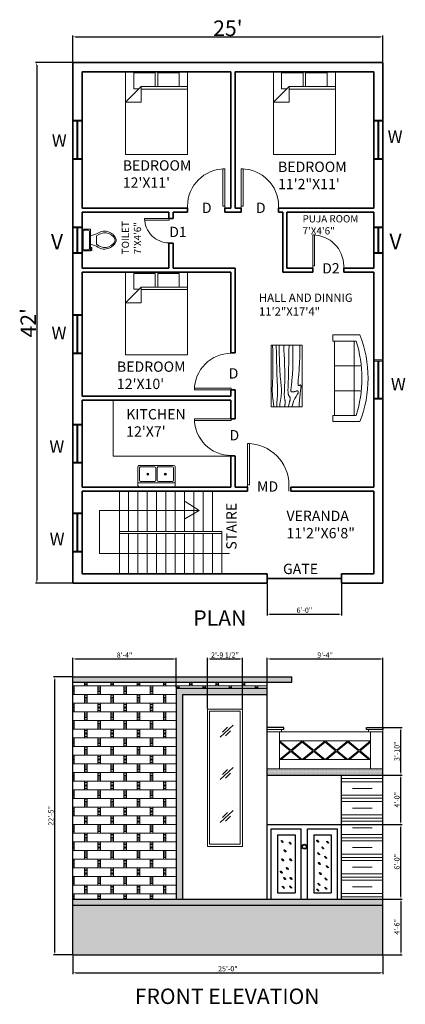
# Model space of a CAD drawing. Units: inches. Extents: x 1662 to 23131, y 1265 to 19127.
# Tile 5 of 26: x 10200 to 10573, y 5334 to 6287. Entities that reach past the tile are written whole.
import ezdxf

# ---------------------------------------------------------------- set-up
doc = ezdxf.new("R2010")
doc.units = ezdxf.units.IN
for name, color, linetype, lineweight in [('A-ANNO-DIMS', 4, 'Continuous', 18), ('A-ANNO-IDEN', 7, 'Continuous', 18), ('A-ANNO-TITL', 7, 'Continuous', 35), ('A-AREA-IDEN', 7, 'Continuous', 18), ('A-DOOR', 3, 'Continuous', 18), ('A-ELEV', 7, 'Continuous', 25), ('A-ELEV-GLAZ', 4, 'Continuous', 18), ('A-ELEV-PATT', 8, 'Continuous', 13), ('A-ELEV-RAIL', 7, 'Continuous', 18), ('A-ELEV-SURF-PATT', 252, 'Continuous', 13), ('A-FLOR-CASE', 8, 'Continuous', 18), ('A-FLOR-FIXT', 9, 'Continuous', 18), ('A-FLOR-STRS', 7, 'Continuous', 18), ('A-FURN', 8, 'Continuous', 18), ('A-GLAZ', 4, 'Continuous', 18), ('A-WALL', 7, 'Continuous', 35)]:
    doc.layers.add(name, color=color, linetype=linetype, lineweight=lineweight)
doc.styles.get("Standard").update_dxf_attribs({"font": 'arial.ttf'})
doc.dimstyles.new('ISO-25', dxfattribs={"dimtxt": 5, "dimasz": 2.5, "dimexe": 1.25, "dimexo": 0.625, "dimtad": 1, "dimlunit": 3, "dimtxsty": 'Standard', "dimcen": 2.5, "dimadec": 0, "dimazin": 0, "dimtfac": 1, "dimtmove": 0, "dimatfit": 3, "dimfxl": 1, "dimarcsym": 0})
pattern_1 = [(0, (-2241.2752, 386.7928), (0.79375, 1.5875), [0, -1.5875])]

# ---------------------------------------------------------------- blocks, each defined once
blk = doc.blocks.new('Bed - Queen')
for p, q in [((0, -80.00003), (0, 0)), ((0, 0), (59.99999, 0)), ((59.99999, 0), (59.99999, -80.00003)), ((7.99999, -1.2), (28.79998, -1.2)), ((7.99999, -14.4), (7.99999, -1.2)), ((28.79998, -1.2), (28.79998, -14.4)), ((31.19999, -1.2), (51.99999, -1.2)), ((31.19999, -14.4), (31.19999, -1.2)), ((51.99999, -1.2), (51.99999, -16.4)), ((0, -14.4), (44.8, -14.4)), ((44.8, -16.8), (0, -16.8)), ((59.99999, -29.6), (44.8, -14.4)), ((44.8, -14.4), (44.8, -29.6)), ((51.99999, -16.4), (46.79936, -16.4)), ((44.8, -29.6), (59.99999, -29.6)), ((59.99999, -80.00003), (0, -80.00003))]:
    blk.add_line(p, q)
blk = doc.blocks.new('Table - Rectangular Woodgrain 60 x 30 in.')
for p, q in [((0, 0), (0, -30)), ((60, 0), (0, 0)), ((60, -30), (60, 0)), ((0, -30), (60, -30))]:
    blk.add_line(p, q)
for points in [[(0, -2.4), (4.8155, -2.418), (9.0302, -2.4688), (12.709, -2.5477), (15.9167, -2.65), (18.7181, -2.7711), (21.1781, -2.9063), (23.3616, -3.0508), (25.3333, -3.2), (27.1477, -3.3495), (28.8172, -3.4958), (30.3437, -3.636), (31.7291, -3.7667), (32.9756, -3.8849), (34.0849, -3.9875), (35.059, -4.0714), (35.9, -4.1334), (36.6114, -4.1711), (37.2041, -4.1854), (37.6906, -4.1779), (38.0833, -4.15), (38.3948, -4.1034), (38.6375, -4.0396), (38.8239, -3.9602), (38.9666, -3.8667), (39.0764, -3.7608), (39.1573, -3.6448), (39.2116, -3.521), (39.2416, -3.3917), (39.2498, -3.2593), (39.2385, -3.1261), (39.21, -2.9944), (39.1666, -2.8667), (39.111, -2.7447), (39.0468, -2.6281), (38.978, -2.5163), (38.9083, -2.4083), (38.8418, -2.3035), (38.7823, -2.201), (38.7337, -2.1001), (38.7, -2), (38.6844, -1.9003), (38.6875, -1.8021), (38.7094, -1.707), (38.75, -1.6167), (38.8094, -1.5326), (38.8875, -1.4563), (38.9844, -1.3893), (39.1, -1.3333), (39.2351, -1.2896), (39.3937, -1.2583), (39.5804, -1.2396), (39.8, -1.2333), (40.057, -1.2396), (40.3562, -1.2583), (40.7023, -1.2896), (41.1, -1.3333), (41.5547, -1.3895), (42.0755, -1.4573), (42.6721, -1.5361), (43.3542, -1.625), (44.1316, -1.7233), (45.014, -1.8302), (46.0114, -1.9449), (47.1333, -2.0667), (48.3862, -2.1947), (49.7625, -2.3281), (51.2513, -2.4663), (52.8416, -2.6083), (54.5226, -2.7535), (56.2833, -2.9011), (58.1127, -3.0501), (60, -3.2)], [(0, -9.2), (6.5759, -9.0858), (11.9385, -9.0365), (16.2527, -9.0418), (19.6833, -9.0917), (22.3952, -9.1759), (24.5531, -9.2844), (26.322, -9.4069), (27.8666, -9.5333), (29.3241, -9.6553), (30.7203, -9.7719), (32.0532, -9.8837), (33.3208, -9.9917), (34.5213, -10.0965), (35.6526, -10.199), (36.7128, -10.2999), (37.7, -10.4), (38.6129, -10.4996), (39.4531, -10.5969), (40.223, -10.6895), (40.925, -10.775), (41.5613, -10.8512), (42.1344, -10.9156), (42.6465, -10.966), (43.1, -11), (43.4976, -11.0158), (43.8437, -11.0136), (44.143, -10.9942), (44.4, -10.9583), (44.6195, -10.9069), (44.8062, -10.8406), (44.9648, -10.7603), (45.1, -10.6667), (45.2155, -10.5598), (45.3114, -10.4365), (45.3871, -10.2929), (45.4416, -10.125), (45.4743, -9.929), (45.4844, -9.7011), (45.4709, -9.4371), (45.4333, -9.1333), (45.3716, -8.7883), (45.2896, -8.4104), (45.1919, -8.0107), (45.0833, -7.6), (44.9685, -7.1893), (44.8521, -6.7896), (44.7388, -6.4117), (44.6333, -6.0667), (44.54, -5.7628), (44.4614, -5.4979), (44.4001, -5.2675), (44.3583, -5.0667), (44.3384, -4.8909), (44.3427, -4.7354), (44.3736, -4.5956), (44.4333, -4.4667), (44.5236, -4.3453), (44.6427, -4.2333), (44.7884, -4.1339), (44.9583, -4.05), (45.1501, -3.9849), (45.3614, -3.9417), (45.59, -3.9234), (45.8333, -3.9333), (46.0915, -3.9749), (46.3734, -4.0531), (46.6906, -4.1736), (47.0542, -4.3417), (47.4756, -4.5629), (47.9661, -4.8427), (48.5372, -5.1866), (49.2, -5.6), (49.9676, -6.0844), (50.8594, -6.625), (51.8965, -7.2031), (53.1, -7.8), (54.491, -8.3969), (56.0906, -8.975), (57.9199, -9.5156), (60, -10)], [(0, -12.8), (5.1847, -12.9322), (9.6213, -13.0323), (13.3963, -13.1059), (16.5958, -13.1583), (19.3063, -13.1952), (21.614, -13.2219), (23.6054, -13.2439), (25.3666, -13.2667), (26.9728, -13.2947), (28.4531, -13.3281), (29.8256, -13.3663), (31.1083, -13.4083), (32.3191, -13.4535), (33.476, -13.501), (34.597, -13.5501), (35.7, -13.6), (36.7984, -13.6497), (37.8875, -13.6979), (38.9578, -13.743), (40, -13.7833), (41.0047, -13.8174), (41.9625, -13.8438), (42.864, -13.8607), (43.7, -13.8667), (44.4631, -13.8604), (45.1552, -13.8417), (45.7801, -13.8104), (46.3416, -13.7667), (46.8439, -13.7104), (47.2906, -13.6417), (47.6858, -13.5604), (48.0333, -13.4667), (48.3375, -13.3608), (48.6042, -13.2448), (48.8396, -13.121), (49.05, -12.9917), (49.2417, -12.8593), (49.4208, -12.7261), (49.5937, -12.5944), (49.7667, -12.4667), (49.9452, -12.3451), (50.1323, -12.2313), (50.3303, -12.1268), (50.5416, -12.0333), (50.7686, -11.9524), (51.0135, -11.8854), (51.2788, -11.8341), (51.5666, -11.8), (51.8785, -11.7843), (52.2116, -11.7865), (52.562, -11.8059), (52.926, -11.8417), (53.2998, -11.8931), (53.6795, -11.9594), (54.0614, -12.0397), (54.4416, -12.1333), (54.8223, -12.2401), (55.2293, -12.3625), (55.6942, -12.5037), (56.2489, -12.6667), (56.9251, -12.8547), (57.7545, -13.0708), (58.7689, -13.3182), (60, -13.6)], [(0, -18), (5.124, -17.7273), (9.6609, -17.5057), (13.6705, -17.3303), (17.2125, -17.1958), (20.3467, -17.0973), (23.1328, -17.0297), (25.6307, -16.9878), (27.9, -16.9667), (29.9928, -16.9617), (31.9302, -16.9703), (33.7254, -16.9907), (35.3917, -17.0208), (36.9423, -17.0588), (38.3906, -17.1026), (39.7499, -17.1503), (41.0333, -17.2), (42.2519, -17.2496), (43.4073, -17.2969), (44.4986, -17.3395), (45.525, -17.375), (46.4858, -17.4012), (47.3802, -17.4156), (48.2074, -17.416), (48.9667, -17.4), (49.6583, -17.3662), (50.2872, -17.3167), (50.8595, -17.2547), (51.3812, -17.1833), (51.8584, -17.1057), (52.2971, -17.025), (52.7034, -16.9443), (53.0833, -16.8667), (53.443, -16.7951), (53.789, -16.7313), (54.128, -16.6768), (54.4666, -16.6334), (54.8115, -16.6024), (55.1693, -16.5854), (55.5465, -16.5841), (55.95, -16.6), (56.3828, -16.6337), (56.8346, -16.6823), (57.2915, -16.7418), (57.7396, -16.8084), (58.165, -16.878), (58.5539, -16.9469), (58.8924, -17.0111), (59.1666, -17.0667), (59.3679, -17.1107), (59.5078, -17.1438), (59.6032, -17.1675), (59.6708, -17.1833), (59.7275, -17.193), (59.7901, -17.1979), (59.8753, -17.1998), (60, -17.2)], [(0, -22.4), (8.0098, -22.2501), (14.4094, -22.1011), (19.4168, -21.9535), (23.25, -21.8083), (26.1269, -21.6663), (28.2656, -21.5281), (29.884, -21.3947), (31.2, -21.2667), (32.3967, -21.1448), (33.5172, -21.0292), (34.5697, -20.9198), (35.5625, -20.8167), (36.5037, -20.7198), (37.4015, -20.6292), (38.2642, -20.5448), (39.1, -20.4667), (39.9164, -20.3951), (40.7187, -20.3313), (41.5117, -20.2768), (42.3, -20.2333), (43.0883, -20.2024), (43.8812, -20.1854), (44.6836, -20.1841), (45.5, -20.2), (46.3328, -20.234), (47.1747, -20.2844), (48.0163, -20.3488), (48.8479, -20.425), (49.66, -20.5106), (50.4429, -20.6031), (51.1872, -20.7004), (51.8833, -20.8), (52.5246, -20.8999), (53.1166, -20.9995), (53.6681, -21.0983), (54.1875, -21.1958), (54.6834, -21.2919), (55.1646, -21.3859), (55.6394, -21.4777), (56.1167, -21.5667), (56.6028, -21.6515), (57.0961, -21.7266), (57.5929, -21.7852), (58.0896, -21.8208), (58.5823, -21.8268), (59.0674, -21.7964), (59.5412, -21.723), (60, -21.6)], [(0, -25.2), (8.6355, -25.0504), (15.7026, -24.9031), (21.4049, -24.7606), (25.9458, -24.625), (29.529, -24.4988), (32.3578, -24.3844), (34.6359, -24.284), (36.5667, -24.2), (38.3213, -24.1341), (39.9417, -24.0854), (41.437, -24.0523), (42.8167, -24.0333), (44.0901, -24.0268), (45.2667, -24.0313), (46.3557, -24.0451), (47.3667, -24.0667), (48.309, -24.0947), (49.1928, -24.1287), (50.0284, -24.168), (50.826, -24.2125), (51.5959, -24.2617), (52.3483, -24.3151), (53.0935, -24.3725), (53.8417, -24.4334), (54.6009, -24.497), (55.3699, -24.561), (56.1454, -24.6226), (56.9239, -24.6792), (57.7021, -24.7279), (58.4764, -24.7662), (59.2435, -24.7911), (60, -24.8)], [(0, -28.8), (5.6867, -28.6681), (10.45, -28.5698), (14.407, -28.5012), (17.675, -28.4584), (20.3711, -28.4374), (22.6125, -28.4344), (24.5164, -28.4455), (26.2, -28.4667), (27.762, -28.4947), (29.2276, -28.5281), (30.6033, -28.5663), (31.8958, -28.6084), (33.1118, -28.6535), (34.2578, -28.7011), (35.3405, -28.7501), (36.3666, -28.8), (37.3443, -28.8497), (38.288, -28.8974), (39.2137, -28.9412), (40.1375, -28.9792), (41.0753, -29.0093), (42.0432, -29.0297), (43.0572, -29.0384), (44.1333, -29.0333), (45.2936, -29.0114), (46.5843, -28.9641), (48.0579, -28.8816), (49.7666, -28.7542), (51.7629, -28.5721), (54.0989, -28.3255), (56.8272, -28.0048), (60, -27.6)]]:
    blk.add_lwpolyline(points)
blk = doc.blocks.new('Sofa - Roundback 7 ft.')
for p, q in [((-12.00002, -32.4421), (-12.00003, -6.5971)), ((11.99997, -32.4421), (11.99998, -6.5971)), ((-36.000027, -34), (-36.000027, -11.4696)), ((-35.999844, -13.3819), (35.9998, -13.3819)), ((35.99998, -34), (35.99998, -11.4696)), ((-36.000027, -32.4421), (35.99998, -32.4421))]:
    blk.add_line(p, q)
for points in [[(-36.000027, -34), (-42.000027, -34), (-42.000027, -8)], [(41.99998, -8), (41.99998, -34), (35.99998, -34)]]:
    blk.add_lwpolyline(points)
for centre, radius, start, end in [((0, -114.25), 114.25, 68.43141, 111.5686), ((-0.00001, -127.1968), 121.1968, 72.72033, 107.2797)]:
    blk.add_arc(centre, radius, start, end)
blk = doc.blocks.new('*U34')
for p, q in [((0, 0), (0, -6)), ((-36, 0), (-36, -6))]:
    blk.add_line(p, q)
blk.add_lwpolyline([(0, 0), (0, 36), (-1.75, 36), (-1.75, 0)], close=True)
blk.add_arc((0, 0), 36, 90, 180)
blk = doc.blocks.new('*U46')
for p, q in [((0, 0), (0, -6)), ((36, 0), (36, -6))]:
    blk.add_line(p, q)
blk.add_lwpolyline([(0, 0), (0, 36), (1.75, 36), (1.75, 0)], close=True)
blk.add_arc((0, 0), 36, 0, 90)
blk = doc.blocks.new('*U41')
for p, q in [((0, 0), (0, -100)), ((-900, 0), (-900, -100))]:
    blk.add_line(p, q)
blk.add_lwpolyline([(0, 0), (0, 900), (-43.75, 900), (-43.75, 0)], close=True)
blk.add_arc((0, 0), 900, 90, 180)
blk = doc.blocks.new('*U42')
for p, q in [((0, 0), (0, -100)), ((900, 0), (900, -100))]:
    blk.add_line(p, q)
blk.add_lwpolyline([(0, 0), (0, 900), (43.75, 900), (43.75, 0)], close=True)
blk.add_arc((0, 0), 900, 0, 90)
blk = doc.blocks.new('*U33')
for p, q in [((0, 0), (0, -6)), ((40, 0), (40, -6))]:
    blk.add_line(p, q)
blk.add_lwpolyline([(0, 0), (0, 40), (1.75, 40), (1.75, 0)], close=True)
blk.add_arc((0, 0), 40, 0, 90)
blk = doc.blocks.new('*U47')
for p, q in [((0, 0), (0, -6)), ((30, 0), (30, -6))]:
    blk.add_line(p, q)
blk.add_lwpolyline([(0, 0), (0, 30), (1.75, 30), (1.75, 0)], close=True)
blk.add_arc((0, 0), 30, 0, 90)
blk = doc.blocks.new('*U48')
for p, q in [((0, 0), (0, 100)), ((600, 0), (600, 100))]:
    blk.add_line(p, q)
blk.add_lwpolyline([(0, 0), (0, -600), (43.75, -600), (43.75, 0)], close=True)
blk.add_arc((0, 0), 600, 270, 0)
blk = doc.blocks.new('Toilet - top')
for p, q in [((-10, -8.5), (-8, -8.5)), ((-10, -9.5), (-10, -8.5)), ((-7, -9.5), (-10, -9.5)), ((-8, -8.5), (-8, -8)), ((-7, -8), (-7, -9.5)), ((-4, -8), (-6, -14)), ((4, -8), (6, -14)), ((9.5, -6), (9.5, -2)), ((4, -14), (-4, -14))]:
    blk.add_line(p, q)
blk.add_lwpolyline([(10.5, -8), (10.5, 0), (-10.5, 0), (-10.5, -8)], close=True)
for points in [[(-9.5, -2), (-9.5, -6)], [(8.5, -1), (-8.5, -1)], [(-8.5, -7), (8.5, -7)]]:
    blk.add_lwpolyline(points)
for centre, radius, start, end in [((-8.62, -1.88), 0.884, 81.8699, 188.1301), ((-8.62, -6.12), 0.884, 171.8699, 278.1301), ((8.62, -1.88), 0.884, 351.8699, 98.1301), ((8.62, -6.12), 0.884, 261.8699, 8.1301), ((3.52, -21.58), 12.17, 141.46911, 247.97143), ((4.2, -21.82), 11.33, 136.36773, 238.94682), ((-3.52, -21.58), 12.17, 292.02843, 38.53071), ((-4.2, -21.82), 11.33, 301.05301, 43.63209), ((0, -27.88), 4, 245.73182, 294.26817), ((0, -29), 4, 254.86053, 285.13947)]:
    blk.add_arc(centre, radius, start, end)
blk = doc.blocks.new('Sink-double - 36 in top')
for p, q in [((-18, -4), (18, -4)), ((-0.75, -18.5), (-0.75, -6.5)), ((0.75, -6.5), (0.75, -18.5))]:
    blk.add_line(p, q)
for points in [[(-16.5, 0), (16.5, 0)], [(-18, -19.5), (-18, -1.5)], [(-16.5, -18.5), (-16.5, -6.5)], [(-15.5, -5.5), (-1.75, -5.5)], [(1.75, -5.5), (15.5, -5.5)], [(16.5, -6.5), (16.5, -18.5)], [(18, -1.5), (18, -19.5)], [(16.5, -21), (-16.5, -21)], [(-1.75, -19.5), (-15.5, -19.5)], [(15.5, -19.5), (1.75, -19.5)]]:
    blk.add_lwpolyline(points)
for centre, radius in [((-8.5, -12.5), 1), ((-8.5, -12.5), 0.5), ((8.5, -12.5), 1), ((8.5, -12.5), 0.5)]:
    blk.add_circle(centre, radius)
for centre, radius, start, end in [((-16.5, -1.5), 1.5, 90, 180), ((16.5, -1.5), 1.5, 0, 90), ((-15.5, -6.5), 1, 90, 180), ((-1.75, -6.5), 1, 0, 90), ((1.75, -6.5), 1, 90, 180), ((15.5, -6.5), 1, 0, 90), ((-15.5, -18.5), 1, 180, 270), ((-1.75, -18.5), 1, 270, 0), ((1.75, -18.5), 1, 180, 270), ((15.5, -18.5), 1, 270, 0), ((-16.5, -19.5), 1.5, 180, 270), ((16.5, -19.5), 1.5, 270, 0)]:
    blk.add_arc(centre, radius, start, end)
blk = doc.blocks.new('*D49')
at = {"layer": 'A-ANNO-DIMS', "color": 0, "lineweight": -2, "transparency": 16777216}
for p, q in [((10251.76, 6246.43), (10251.76, 6271.87)), ((10551.76, 6246.43), (10551.76, 6271.87)), ((10254.26, 6270.62), (10549.26, 6270.62))]:
    blk.add_line(p, q, dxfattribs=at)
at = {"layer": 'A-ANNO-DIMS', "color": 0, "transparency": 16777216}
for points in [[(10254.26, 6271.03), (10254.26, 6270.2), (10251.76, 6270.62)], [(10549.26, 6271.03), (10549.26, 6270.2), (10551.76, 6270.62)]]:
    blk.add_solid(points, dxfattribs=at)
at = {"layer": 'Defpoints', "color": 0, "transparency": 16777216}
for p in [(10551.76, 6270.62), (10251.76, 6245.8), (10551.76, 6245.8)]:
    blk.add_point(p, dxfattribs=at)
at = {"layer": 'A-ANNO-DIMS', "color": 0, "transparency": 16777216, "insert": (10401.76, 6278.9), "char_height": 5, "attachment_point": 5}
blk.add_mtext("{\\H3x;25'}", dxfattribs=at)
blk = doc.blocks.new('*D50')
at = {"layer": 'A-ANNO-DIMS', "color": 0, "lineweight": -2, "transparency": 16777216}
for p, q in [((10251.14, 6245.8), (10215.58, 6245.8)), ((10216.83, 6243.3), (10216.83, 5744.3)), ((10251.14, 5741.8), (10215.58, 5741.8))]:
    blk.add_line(p, q, dxfattribs=at)
at = {"layer": 'A-ANNO-DIMS', "color": 0, "transparency": 16777216}
for points in [[(10216.41, 6243.3), (10217.25, 6243.3), (10216.83, 6245.8)], [(10216.41, 5744.3), (10217.25, 5744.3), (10216.83, 5741.8)]]:
    blk.add_solid(points, dxfattribs=at)
at = {"layer": 'Defpoints', "color": 0, "transparency": 16777216}
for p in [(10251.76, 6245.8), (10216.83, 5741.8), (10251.76, 5741.8)]:
    blk.add_point(p, dxfattribs=at)
at = {"layer": 'A-ANNO-DIMS', "color": 0, "transparency": 16777216, "insert": (10208.68, 5993.8), "char_height": 5, "attachment_point": 5, "rotation": 90}
blk.add_mtext("{\\H3x;42'}", dxfattribs=at)
blk = doc.blocks.new('WIN-36-J9X1')
for p, q in [((0, 9), (0, 0)), ((1, 9), (1, 0)), ((1, 5), (37, 5)), ((1, 4.5), (37, 4.5)), ((1, 4), (37, 4)), ((37, 9), (37, 0)), ((38, 9), (38, 0))]:
    blk.add_line(p, q)
blk = doc.blocks.new('VENT-24-J9X1')
for p, q in [((0, 9), (0, 0)), ((1, 9), (1, 0)), ((1, 5), (25, 5)), ((1, 4.5), (25, 4.5)), ((1, 4), (25, 4)), ((25, 9), (25, 0)), ((26, 9), (26, 0))]:
    blk.add_line(p, q)
blk = doc.blocks.new('GLAZ-REFLECTION-TALL')
for p, q in [((0, 0), (12.57, 11.7)), ((2.1, 4.93), (7.03, 9.61)), ((5.05, 1.35), (9.86, 6.16))]:
    blk.add_line(p, q)
blk = doc.blocks.new('*D209')
at = {"layer": 'A-ANNO-DIMS', "color": 0, "lineweight": -2, "transparency": 16777216}
for p, q in [((10439.76, 5741.18), (10439.76, 5710.5)), ((10511.76, 5741.18), (10511.76, 5710.5)), ((10442.26, 5711.75), (10509.26, 5711.75))]:
    blk.add_line(p, q, dxfattribs=at)
at = {"layer": 'A-ANNO-DIMS', "color": 0, "transparency": 16777216}
for points in [[(10442.26, 5712.17), (10442.26, 5711.33), (10439.76, 5711.75)], [(10509.26, 5712.17), (10509.26, 5711.33), (10511.76, 5711.75)]]:
    blk.add_solid(points, dxfattribs=at)
at = {"layer": 'Defpoints', "color": 0, "transparency": 16777216}
for p in [(10439.76, 5741.8), (10511.76, 5741.8), (10511.76, 5711.75)]:
    blk.add_point(p, dxfattribs=at)
at = {"layer": 'A-ANNO-DIMS', "color": 0, "transparency": 16777216, "insert": (10475.76, 5714.93), "char_height": 5, "attachment_point": 5}
blk.add_mtext('6\'-0"', dxfattribs=at)
blk = doc.blocks.new('*D210')
at = {"layer": 'A-ANNO-DIMS', "color": 0, "lineweight": -2, "transparency": 16777216}
for p, q in [((10251.76, 5381.38), (10251.76, 5363.4)), ((10551.76, 5381.38), (10551.76, 5363.4)), ((10254.26, 5364.65), (10549.26, 5364.65))]:
    blk.add_line(p, q, dxfattribs=at)
at = {"layer": 'A-ANNO-DIMS', "color": 0, "transparency": 16777216}
for points in [[(10254.26, 5365.07), (10254.26, 5364.23), (10251.76, 5364.65)], [(10549.26, 5365.07), (10549.26, 5364.23), (10551.76, 5364.65)]]:
    blk.add_solid(points, dxfattribs=at)
at = {"layer": 'Defpoints', "color": 0, "transparency": 16777216}
for p in [(10251.76, 5382), (10551.76, 5382), (10551.76, 5364.65)]:
    blk.add_point(p, dxfattribs=at)
at = {"layer": 'A-ANNO-DIMS', "color": 0, "transparency": 16777216, "insert": (10401.76, 5367.83), "char_height": 5, "attachment_point": 5}
blk.add_mtext('25\'-0"', dxfattribs=at)
blk = doc.blocks.new('*D211')
at = {"layer": 'A-ANNO-DIMS', "color": 0, "lineweight": -2, "transparency": 16777216}
for p, q in [((10251.14, 5651), (10233.16, 5651)), ((10234.41, 5384.5), (10234.41, 5648.5)), ((10251.14, 5382), (10233.16, 5382))]:
    blk.add_line(p, q, dxfattribs=at)
at = {"layer": 'A-ANNO-DIMS', "color": 0, "transparency": 16777216}
for points in [[(10234, 5648.5), (10234.83, 5648.5), (10234.41, 5651)], [(10234, 5384.5), (10234.83, 5384.5), (10234.41, 5382)]]:
    blk.add_solid(points, dxfattribs=at)
at = {"layer": 'Defpoints', "color": 0, "transparency": 16777216}
for p in [(10234.41, 5651), (10251.76, 5651), (10251.76, 5382)]:
    blk.add_point(p, dxfattribs=at)
at = {"layer": 'A-ANNO-DIMS', "color": 0, "transparency": 16777216, "insert": (10231.23, 5516.5), "char_height": 5, "attachment_point": 5, "rotation": 90}
blk.add_mtext('22\'-5"', dxfattribs=at)
blk = doc.blocks.new('*D212')
at = {"layer": 'A-ANNO-DIMS', "color": 0, "lineweight": -2, "transparency": 16777216}
for p, q in [((10552.39, 5436), (10570.36, 5436)), ((10569.11, 5433.5), (10569.11, 5384.5)), ((10552.39, 5382), (10570.36, 5382))]:
    blk.add_line(p, q, dxfattribs=at)
at = {"layer": 'A-ANNO-DIMS', "color": 0, "transparency": 16777216}
for points in [[(10568.7, 5433.5), (10569.53, 5433.5), (10569.11, 5436)], [(10568.7, 5384.5), (10569.53, 5384.5), (10569.11, 5382)]]:
    blk.add_solid(points, dxfattribs=at)
at = {"layer": 'Defpoints', "color": 0, "transparency": 16777216}
for p in [(10551.76, 5436), (10551.76, 5382), (10569.11, 5382)]:
    blk.add_point(p, dxfattribs=at)
at = {"layer": 'A-ANNO-DIMS', "color": 0, "transparency": 16777216, "insert": (10565.93, 5409), "char_height": 5, "attachment_point": 5, "rotation": 90}
blk.add_mtext('4\'-6"', dxfattribs=at)
blk = doc.blocks.new('*D213')
at = {"layer": 'A-ANNO-DIMS', "color": 0, "lineweight": -2, "transparency": 16777216}
for p, q in [((10512.39, 5508), (10570.36, 5508)), ((10569.11, 5438.5), (10569.11, 5505.5)), ((10512.39, 5436), (10570.36, 5436))]:
    blk.add_line(p, q, dxfattribs=at)
at = {"layer": 'A-ANNO-DIMS', "color": 0, "transparency": 16777216}
for points in [[(10568.7, 5505.5), (10569.53, 5505.5), (10569.11, 5508)], [(10568.7, 5438.5), (10569.53, 5438.5), (10569.11, 5436)]]:
    blk.add_solid(points, dxfattribs=at)
at = {"layer": 'Defpoints', "color": 0, "transparency": 16777216}
for p in [(10511.76, 5508), (10569.11, 5508), (10511.76, 5436)]:
    blk.add_point(p, dxfattribs=at)
at = {"layer": 'A-ANNO-DIMS', "color": 0, "transparency": 16777216, "insert": (10565.93, 5472), "char_height": 5, "attachment_point": 5, "rotation": 90}
blk.add_mtext('6\'-0"', dxfattribs=at)
blk = doc.blocks.new('*D214')
at = {"layer": 'A-ANNO-DIMS', "color": 0, "lineweight": -2, "transparency": 16777216}
for p, q in [((10552.39, 5556), (10570.36, 5556)), ((10569.11, 5510.5), (10569.11, 5553.5)), ((10512.39, 5508), (10570.36, 5508))]:
    blk.add_line(p, q, dxfattribs=at)
at = {"layer": 'A-ANNO-DIMS', "color": 0, "transparency": 16777216}
for points in [[(10568.7, 5553.5), (10569.53, 5553.5), (10569.11, 5556)], [(10568.7, 5510.5), (10569.53, 5510.5), (10569.11, 5508)]]:
    blk.add_solid(points, dxfattribs=at)
at = {"layer": 'Defpoints', "color": 0, "transparency": 16777216}
for p in [(10551.76, 5556), (10569.11, 5556), (10511.76, 5508)]:
    blk.add_point(p, dxfattribs=at)
at = {"layer": 'A-ANNO-DIMS', "color": 0, "transparency": 16777216, "insert": (10565.93, 5532), "char_height": 5, "attachment_point": 5, "rotation": 90}
blk.add_mtext('4\'-0"', dxfattribs=at)
blk = doc.blocks.new('*D215')
at = {"layer": 'A-ANNO-DIMS', "color": 0, "lineweight": -2, "transparency": 16777216}
for p, q in [((10552.39, 5602), (10570.36, 5602)), ((10569.11, 5558.5), (10569.11, 5599.5)), ((10552.39, 5556), (10570.36, 5556))]:
    blk.add_line(p, q, dxfattribs=at)
at = {"layer": 'A-ANNO-DIMS', "color": 0, "transparency": 16777216}
for points in [[(10568.7, 5599.5), (10569.53, 5599.5), (10569.11, 5602)], [(10568.7, 5558.5), (10569.53, 5558.5), (10569.11, 5556)]]:
    blk.add_solid(points, dxfattribs=at)
at = {"layer": 'Defpoints', "color": 0, "transparency": 16777216}
for p in [(10551.76, 5602), (10569.11, 5602), (10551.76, 5556)]:
    blk.add_point(p, dxfattribs=at)
at = {"layer": 'A-ANNO-DIMS', "color": 0, "transparency": 16777216, "insert": (10565.93, 5579), "char_height": 5, "attachment_point": 5, "rotation": 90}
blk.add_mtext('3\'-10"', dxfattribs=at)
blk = doc.blocks.new('*D216')
at = {"layer": 'A-ANNO-DIMS', "color": 0, "lineweight": -2, "transparency": 16777216}
for p, q in [((10251.76, 5646.63), (10251.76, 5669.6)), ((10254.26, 5668.35), (10349.26, 5668.35)), ((10351.76, 5640.63), (10351.76, 5669.6))]:
    blk.add_line(p, q, dxfattribs=at)
at = {"layer": 'A-ANNO-DIMS', "color": 0, "transparency": 16777216}
for points in [[(10254.26, 5668.77), (10254.26, 5667.93), (10251.76, 5668.35)], [(10349.26, 5668.77), (10349.26, 5667.93), (10351.76, 5668.35)]]:
    blk.add_solid(points, dxfattribs=at)
at = {"layer": 'Defpoints', "color": 0, "transparency": 16777216}
for p in [(10351.76, 5668.35), (10251.76, 5646), (10351.76, 5640)]:
    blk.add_point(p, dxfattribs=at)
at = {"layer": 'A-ANNO-DIMS', "color": 0, "transparency": 16777216, "insert": (10301.76, 5671.53), "char_height": 5, "attachment_point": 5}
blk.add_mtext('8\'-4"', dxfattribs=at)
blk = doc.blocks.new('*D217')
at = {"layer": 'A-ANNO-DIMS', "color": 0, "lineweight": -2, "transparency": 16777216}
for p, q in [((10382.08, 5620.39), (10382.08, 5669.6)), ((10384.58, 5668.35), (10413.26, 5668.35)), ((10415.76, 5620.39), (10415.76, 5669.6))]:
    blk.add_line(p, q, dxfattribs=at)
at = {"layer": 'A-ANNO-DIMS', "color": 0, "transparency": 16777216}
for points in [[(10384.58, 5668.77), (10384.58, 5667.93), (10382.08, 5668.35)], [(10413.26, 5668.77), (10413.26, 5667.93), (10415.76, 5668.35)]]:
    blk.add_solid(points, dxfattribs=at)
at = {"layer": 'Defpoints', "color": 0, "transparency": 16777216}
for p in [(10415.76, 5668.35), (10382.08, 5619.77), (10415.76, 5619.77)]:
    blk.add_point(p, dxfattribs=at)
at = {"layer": 'A-ANNO-DIMS', "color": 0, "transparency": 16777216, "insert": (10398.92, 5671.56), "char_height": 5, "attachment_point": 5}
blk.add_mtext('2\'-9 1/2"', dxfattribs=at)
blk = doc.blocks.new('*D218')
at = {"layer": 'A-ANNO-DIMS', "color": 0, "lineweight": -2, "transparency": 16777216}
for p, q in [((10439.76, 5600.63), (10439.76, 5669.6)), ((10442.26, 5668.35), (10549.26, 5668.35)), ((10551.76, 5600.63), (10551.76, 5669.6))]:
    blk.add_line(p, q, dxfattribs=at)
at = {"layer": 'A-ANNO-DIMS', "color": 0, "transparency": 16777216}
for points in [[(10442.26, 5668.77), (10442.26, 5667.93), (10439.76, 5668.35)], [(10549.26, 5668.77), (10549.26, 5667.93), (10551.76, 5668.35)]]:
    blk.add_solid(points, dxfattribs=at)
at = {"layer": 'Defpoints', "color": 0, "transparency": 16777216}
for p in [(10551.76, 5668.35), (10439.76, 5600), (10551.76, 5600)]:
    blk.add_point(p, dxfattribs=at)
at = {"layer": 'A-ANNO-DIMS', "color": 0, "transparency": 16777216, "insert": (10495.76, 5671.53), "char_height": 5, "attachment_point": 5}
blk.add_mtext('9\'-4"', dxfattribs=at)

msp = doc.modelspace()

# ---------------------------------------------------------------- hatches: boundary and pattern name
at = {"layer": 'A-ELEV-PATT'}
h = msp.add_hatch(dxfattribs=at)
h.set_pattern_fill('BRSTONE', color=256)
h.set_pattern_definition([(0, (-2241.275, 386.793), (0, 8.382), []), (90, (-2218.415, 386.793), (-12.7, 8.382), [8.382, -8.382]), (90, (-2220.955, 386.793), (-12.7, 8.382), [8.382, -8.382]), (0, (-2218.415, 388.19), (12.7, 8.382), [-22.86, 2.54]), (0, (-2218.415, 389.587), (12.7, 8.382), [-22.86, 2.54]), (0, (-2218.415, 390.984), (12.7, 8.382), [-22.86, 2.54]), (0, (-2218.415, 392.381), (12.7, 8.382), [-22.86, 2.54]), (0, (-2218.415, 393.778), (12.7, 8.382), [-22.86, 2.54])])
h.paths.add_polyline_path([(10351.762, 5640), (10439.762, 5640), (10439.762, 5646), (10251.762, 5646), (10251.762, 5436), (10351.762, 5436)])
h = msp.add_hatch(dxfattribs=at)
h.set_pattern_fill('DOTS', color=256)
h.set_pattern_definition(pattern_1)
h.paths.add_polyline_path([(10351.762, 5436), (10357.762, 5436), (10357.762, 5634), (10439.762, 5634), (10439.762, 5640), (10351.762, 5640)])
h = msp.add_hatch(dxfattribs=at)
h.set_pattern_fill('DOTS', color=256)
h.set_pattern_definition(pattern_1)
h.paths.add_polyline_path([(10551.762, 5556), (10551.762, 5562), (10439.762, 5562), (10439.762, 5556)])
h = msp.add_hatch(dxfattribs=at)
h.set_pattern_fill('CLAY', color=256, scale=4)
h.set_pattern_definition([(0, (-2241.275, 386.793), (0, 19.05), []), (0, (-2241.275, 389.968), (0, 19.05), []), (0, (-2241.275, 393.143), (0, 19.05), []), (0, (-2241.275, 399.493), (0, 19.05), [19.05, -12.7])])
h.paths.add_polyline_path([(10511.762, 5436), (10551.762, 5436), (10551.762, 5556), (10511.762, 5556)])
h = msp.add_hatch(dxfattribs=at)
h.set_pattern_fill('DOTS', color=256)
h.set_pattern_definition(pattern_1)
h.paths.add_polyline_path([(10551.762, 5430), (10551.762, 5436), (10251.762, 5436), (10251.762, 5430)])
at = {"layer": 'A-ELEV-SURF-PATT'}
h = msp.add_hatch(color=256, dxfattribs=at)
h.dxf.hatch_style = 1
h.paths.add_polyline_path([(10251.762, 5651), (10251.762, 5646), (10463.762, 5646), (10463.762, 5651)])
h.paths.add_polyline_path([(10551.762, 5556), (10551.762, 5562), (10439.762, 5562), (10439.762, 5556)])
h = msp.add_hatch(color=256, dxfattribs=at)
h.dxf.hatch_style = 1
h.paths.add_polyline_path([(10551.762, 5382), (10551.762, 5430), (10251.762, 5430), (10251.762, 5382)])

# ---------------------------------------------------------------- linework, layer by layer
at = {"layer": 'A-ELEV'}
for p, q in [((10251.762, 5382), (10251.762, 5651)), ((10251.762, 5651), (10463.762, 5651)), ((10251.762, 5646), (10463.762, 5646)), ((10439.762, 5436), (10439.762, 5646)), ((10463.762, 5646), (10463.762, 5651)), ((10351.762, 5640), (10439.762, 5640)), ((10351.762, 5640), (10351.762, 5436)), ((10357.762, 5634), (10439.762, 5634)), ((10357.762, 5634), (10357.762, 5436)), ((10455.762, 5602), (10439.762, 5602)), ((10455.762, 5600), (10455.762, 5602)), ((10535.762, 5600), (10535.762, 5602)), ((10535.762, 5602), (10551.762, 5602)), ((10551.762, 5602), (10551.762, 5600)), ((10551.762, 5382), (10551.762, 5598)), ((10439.762, 5556), (10551.762, 5556)), ((10511.762, 5436), (10511.762, 5556)), ((10439.762, 5508), (10511.762, 5508)), ((10443.762, 5436), (10443.762, 5504)), ((10443.762, 5504), (10472.762, 5504)), ((10472.762, 5436), (10472.762, 5504)), ((10478.762, 5436), (10478.762, 5504)), ((10478.762, 5504), (10507.762, 5504)), ((10507.762, 5436), (10507.762, 5504)), ((10449.762, 5498), (10466.762, 5498)), ((10449.762, 5498), (10449.762, 5442)), ((10466.762, 5498), (10466.762, 5442)), ((10484.762, 5498), (10501.762, 5498)), ((10484.762, 5498), (10484.762, 5442)), ((10501.762, 5498), (10501.762, 5442)), ((10251.762, 5436), (10551.762, 5436)), ((10449.762, 5442), (10466.762, 5442)), ((10484.762, 5442), (10501.762, 5442)), ((10251.762, 5430), (10551.762, 5430)), ((10251.762, 5382), (10551.762, 5382))]:
    msp.add_line(p, q, dxfattribs=at)
for radius in [2.405, 1.831]:
    msp.add_circle((10475.762, 5486.654), radius, dxfattribs=at)
for centre in [(10454.229, 5491.685), (10461.984, 5490.025), (10488.702, 5492.064), (10498.313, 5490.962), (10456.937, 5482.647), (10489.49, 5479.945), (10493.586, 5485.453), (10454.671, 5473.964), (10462.548, 5473.964), (10490.278, 5470.343), (10496.265, 5476.324), (10453.568, 5462.002), (10459.24, 5465.622), (10491.066, 5460.742), (10497.84, 5467.353), (10456.561, 5455.863), (10462.863, 5455.863), (10496.58, 5455.391), (10455.458, 5447.364), (10462.391, 5447.679), (10488.686, 5444.68), (10489.805, 5450.197), (10496.58, 5446.419)]:
    msp.add_ellipse(centre, major_axis=(0.776, -1.013), ratio=0.2977861, start_param=-3.141592653589793, end_param=3.141592653589793, dxfattribs=at)
at = {"layer": 'A-ELEV-GLAZ'}
for points in [[(10382.08, 5619.768), (10415.759, 5619.768), (10415.759, 5486.963), (10382.08, 5486.963)], [(10384.08, 5617.768), (10413.759, 5617.768), (10413.759, 5488.963), (10384.08, 5488.963)]]:
    msp.add_lwpolyline(points, close=True, dxfattribs=at)
at = {"layer": 'A-ELEV-RAIL'}
for p, q in [((10453.762, 5600), (10439.762, 5600)), ((10439.762, 5598), (10551.762, 5598)), ((10451.762, 5562), (10451.762, 5598)), ((10451.762, 5598), (10453.762, 5598)), ((10453.762, 5598), (10453.762, 5600)), ((10453.762, 5600), (10455.762, 5600)), ((10537.762, 5600), (10535.762, 5600)), ((10537.762, 5598), (10537.762, 5600)), ((10537.762, 5600), (10551.762, 5600)), ((10539.762, 5598), (10537.762, 5598)), ((10539.762, 5562), (10539.762, 5598)), ((10551.762, 5600), (10551.762, 5598)), ((10451.762, 5589), (10539.762, 5589)), ((10462.762, 5580), (10451.762, 5589)), ((10461.972, 5579.354), (10451.762, 5587.708)), ((10462.762, 5580), (10473.762, 5589)), ((10463.551, 5579.354), (10473.762, 5587.708)), ((10473.762, 5589), (10484.762, 5580)), ((10473.762, 5587.708), (10483.972, 5579.354)), ((10495.762, 5589), (10484.762, 5580)), ((10495.762, 5587.708), (10485.551, 5579.354)), ((10506.762, 5580), (10495.762, 5589)), ((10505.972, 5579.354), (10495.762, 5587.708)), ((10506.762, 5580), (10517.762, 5589)), ((10507.551, 5579.354), (10517.762, 5587.708)), ((10517.762, 5589), (10528.762, 5580)), ((10517.762, 5587.708), (10527.972, 5579.354)), ((10539.762, 5589), (10528.762, 5580)), ((10539.762, 5587.708), (10529.551, 5579.354)), ((10451.762, 5571), (10461.972, 5579.354)), ((10453.341, 5571), (10462.762, 5578.708)), ((10472.183, 5571), (10462.762, 5578.708)), ((10473.762, 5571), (10463.551, 5579.354)), ((10483.972, 5579.354), (10473.762, 5571)), ((10484.762, 5578.708), (10475.341, 5571)), ((10484.762, 5578.708), (10494.183, 5571)), ((10485.551, 5579.354), (10495.762, 5571)), ((10495.762, 5571), (10505.972, 5579.354)), ((10497.341, 5571), (10506.762, 5578.708)), ((10516.183, 5571), (10506.762, 5578.708)), ((10517.762, 5571), (10507.551, 5579.354)), ((10527.972, 5579.354), (10517.762, 5571)), ((10528.762, 5578.708), (10519.341, 5571)), ((10528.762, 5578.708), (10538.183, 5571)), ((10529.551, 5579.354), (10539.762, 5571)), ((10451.762, 5571), (10539.762, 5571)), ((10439.762, 5562), (10551.762, 5562))]:
    msp.add_line(p, q, dxfattribs=at)
at = {"layer": 'A-FLOR-CASE'}
for q in [(10290.762, 5918.801), (10408.762, 5864.801)]:
    msp.add_line((10290.762, 5864.801), q, dxfattribs=at)
at = {"layer": 'A-FLOR-STRS'}
for p, q in [((10296.762, 5750.801), (10296.762, 5830.801)), ((10305.762, 5791.801), (10305.762, 5830.801)), ((10314.762, 5791.801), (10314.762, 5830.801)), ((10323.762, 5791.801), (10323.762, 5830.801)), ((10332.762, 5791.801), (10332.762, 5830.801)), ((10341.762, 5791.801), (10341.762, 5830.801)), ((10350.762, 5791.801), (10350.762, 5830.801)), ((10359.762, 5791.801), (10359.762, 5830.801)), ((10368.762, 5791.801), (10368.762, 5830.801)), ((10377.762, 5791.801), (10377.762, 5830.801)), ((10377.762, 5791.801), (10377.762, 5830.801)), ((10386.762, 5791.801), (10386.762, 5830.801)), ((10373.855, 5812.178), (10360.47, 5820.799)), ((10277.676, 5770.359), (10277.676, 5812.178)), ((10277.676, 5812.178), (10373.855, 5812.178)), ((10373.855, 5812.178), (10360.222, 5803.874)), ((10296.762, 5791.801), (10395.762, 5791.801)), ((10296.762, 5789.801), (10395.762, 5789.801)), ((10305.762, 5750.801), (10305.762, 5789.801)), ((10314.762, 5750.801), (10314.762, 5789.801)), ((10323.762, 5750.801), (10323.762, 5789.801)), ((10332.762, 5750.801), (10332.762, 5789.801)), ((10341.762, 5750.801), (10341.762, 5789.801)), ((10350.762, 5750.801), (10350.762, 5789.801)), ((10359.762, 5750.801), (10359.762, 5789.801)), ((10368.762, 5750.801), (10368.762, 5789.801)), ((10377.762, 5750.801), (10377.762, 5789.801)), ((10377.762, 5750.801), (10377.762, 5789.801)), ((10386.762, 5750.801), (10386.762, 5789.801)), ((10395.762, 5750.801), (10395.762, 5791.801)), ((10403.349, 5770.359), (10277.676, 5770.359))]:
    msp.add_line(p, q, dxfattribs=at)
at = {"layer": 'A-WALL'}
for p, q in [((10251.762, 6245.801), (10551.762, 6245.801)), ((10251.762, 5741.801), (10251.762, 6245.801)), ((10551.762, 6245.801), (10551.762, 5741.801)), ((10260.762, 6236.801), (10404.762, 6236.801)), ((10260.762, 6104.801), (10260.762, 6236.801)), ((10404.762, 6104.801), (10404.762, 6236.801)), ((10408.762, 6104.801), (10408.762, 6236.801)), ((10408.762, 6236.801), (10542.762, 6236.801)), ((10542.762, 6236.801), (10542.762, 6104.801)), ((10260.762, 6104.801), (10362.762, 6104.801)), ((10260.762, 6100.801), (10344.762, 6100.801)), ((10260.762, 6046.801), (10260.762, 6100.801)), ((10344.762, 6094.801), (10344.762, 6100.801)), ((10348.762, 6094.801), (10348.762, 6100.801)), ((10348.762, 6100.801), (10362.762, 6100.801)), ((10362.762, 6100.801), (10362.762, 6104.801)), ((10398.762, 6100.801), (10398.762, 6104.801)), ((10398.762, 6104.801), (10404.762, 6104.801)), ((10398.762, 6100.801), (10414.762, 6100.801)), ((10408.762, 6104.801), (10414.762, 6104.801)), ((10414.762, 6100.801), (10414.762, 6104.801)), ((10450.762, 6100.801), (10450.762, 6104.801)), ((10450.762, 6104.801), (10542.762, 6104.801)), ((10450.762, 6100.801), (10454.762, 6100.801)), ((10454.762, 6100.801), (10454.762, 6042.801)), ((10458.762, 6100.801), (10458.762, 6046.801)), ((10458.762, 6100.801), (10542.762, 6100.801)), ((10542.762, 6100.801), (10542.762, 6046.801)), ((10344.762, 6094.801), (10348.762, 6094.801)), ((10344.762, 6046.801), (10344.762, 6070.801)), ((10344.762, 6070.801), (10348.762, 6070.801)), ((10348.762, 6046.801), (10348.762, 6070.801)), ((10260.762, 6046.801), (10344.762, 6046.801)), ((10260.762, 6042.801), (10404.762, 6042.801)), ((10260.762, 5922.801), (10260.762, 6042.801)), ((10348.762, 6046.801), (10408.762, 6046.801)), ((10404.762, 5964.801), (10404.762, 6042.801)), ((10408.762, 5964.801), (10408.762, 6046.801)), ((10454.762, 6042.801), (10483.762, 6042.801)), ((10458.762, 6046.801), (10483.762, 6046.801)), ((10483.762, 6042.801), (10483.762, 6046.801)), ((10513.762, 6042.801), (10513.762, 6046.801)), ((10513.762, 6046.801), (10542.762, 6046.801)), ((10513.762, 6042.801), (10542.762, 6042.801)), ((10542.762, 6042.801), (10542.762, 5834.801)), ((10404.762, 5964.801), (10408.762, 5964.801)), ((10404.762, 5922.801), (10404.762, 5928.801)), ((10404.762, 5928.801), (10408.762, 5928.801)), ((10408.762, 5900.801), (10408.762, 5928.801)), ((10260.762, 5922.801), (10404.762, 5922.801)), ((10260.762, 5918.801), (10404.762, 5918.801)), ((10260.762, 5834.801), (10260.762, 5918.801)), ((10404.762, 5900.801), (10404.762, 5918.801)), ((10404.762, 5900.801), (10408.762, 5900.801)), ((10404.762, 5834.801), (10404.762, 5864.801)), ((10408.762, 5834.801), (10408.762, 5864.801)), ((10260.762, 5834.801), (10404.762, 5834.801)), ((10408.762, 5834.801), (10420.762, 5834.801)), ((10420.762, 5834.801), (10420.762, 5830.801)), ((10462.762, 5834.801), (10462.762, 5830.801)), ((10462.762, 5834.801), (10542.762, 5834.801)), ((10260.762, 5750.801), (10260.762, 5830.801)), ((10260.762, 5830.801), (10420.762, 5830.801)), ((10462.762, 5830.801), (10542.762, 5830.801)), ((10542.762, 5830.801), (10542.762, 5750.801)), ((10439.762, 5750.801), (10260.762, 5750.801)), ((10439.762, 5750.801), (10439.762, 5741.801)), ((10542.762, 5750.801), (10511.762, 5750.801)), ((10511.762, 5750.801), (10511.762, 5741.801)), ((10439.762, 5741.801), (10251.762, 5741.801)), ((10439.762, 5746.301), (10511.762, 5746.301)), ((10551.762, 5741.801), (10511.762, 5741.801))]:
    msp.add_line(p, q, dxfattribs=at)

# ---------------------------------------------------------------- block references
at = {"layer": 'A-DOOR'}
for name, p in [('*U34', (10398.762, 6106.801)), ('*U46', (10414.762, 6106.801)), ('*U47', (10483.762, 6048.801)), ('*U33', (10420.762, 5836.801))]:
    msp.add_blockref(name, p, dxfattribs=at)
at = {"layer": 'A-DOOR', "xscale": 0.0393700787401575, "yscale": 0.0393700787401575, "zscale": 0.0393700787401575}
for name, p, rotation in [('*U48', (10344.825, 6094.801), 270), ('*U42', (10404.825, 5928.801), 89.99999999999996), ('*U41', (10404.825, 5900.801), 89.99999999999996)]:
    msp.add_blockref(name, p, dxfattribs=dict(at, rotation=rotation))
at = {"layer": 'A-ELEV-GLAZ'}
for p in [(10394.389, 5592.704), (10394.389, 5551.743), (10394.389, 5510.025)]:
    msp.add_blockref('GLAZ-REFLECTION-TALL', p, dxfattribs=at)
at = {"layer": 'A-FLOR-FIXT'}
for name, p, rotation in [('Toilet - top', (10260.762, 6073.801), 89.99999999999999), ('Sink-double - 36 in top', (10332.762, 5834.801), 180)]:
    msp.add_blockref(name, p, dxfattribs=dict(at, rotation=rotation))
at = {"layer": 'A-FURN', "xscale": -1}
for p in [(10362.762, 6236.801), (10505.762, 6236.801), (10362.762, 6042.801)]:
    msp.add_blockref('Bed - Queen', p, dxfattribs=at)
at = {"layer": 'A-FURN'}
for name, p, rotation in [('Sofa - Roundback 7 ft.', (10537.347, 5940.079), 269.9999999999999), ('Table - Rectangular Woodgrain 60 x 30 in.', (10473.752, 5972.282), 270)]:
    msp.add_blockref(name, p, dxfattribs=dict(at, rotation=rotation))
at = {"layer": 'A-GLAZ', "rotation": 90}
for name, p in [('WIN-36-J9X1', (10260.762, 6151.801)), ('WIN-36-J9X1', (10551.762, 6151.801)), ('VENT-24-J9X1', (10260.762, 6060.801)), ('VENT-24-J9X1', (10551.762, 6060.801)), ('WIN-36-J9X1', (10260.762, 5963.801)), ('WIN-36-J9X1', (10551.762, 5919.801)), ('WIN-36-J9X1', (10260.762, 5857.801)), ('WIN-36-J9X1', (10260.762, 5771.801))]:
    msp.add_blockref(name, p, dxfattribs=at)

# ---------------------------------------------------------------- texts
at = {"layer": 'A-ANNO-IDEN', "attachment_point": 1}
for s, width, heights, insert, char_height in [('W', 471.52273, [28.462], (10231.481, 6176.272), 12), ('W', 471.52273, [28.462], (10556.316, 6179.946), 12), ('D', 1142.59551, [0], (10376.623, 6110.078), 10), ('D', 1142.59551, [0], (10428.869, 6110.078), 10), ('D1', 1142.59551, [20], (10345, 6086.754), 10), ('V', 1142.59551, [20], (10230.57, 6079.807), 15), ('V', 1142.59551, [20], (10558.01, 6079.988), 15), ('D2', 1142.59551, [20], (10492.926, 6051.501), 10), ('W', 471.52273, [28.462], (10231.226, 5989.888), 12), ('D', 1142.59551, [0], (10402.515, 5949.811), 10), ('W', 471.52273, [28.462], (10559.419, 5940.333), 12), ('D', 1142.59551, [0], (10403.309, 5889.925), 10), ('W', 471.52273, [28.462], (10229.1, 5880.009), 12), ('MD', 1142.59551, [0], (10429.909, 5840.324), 10), ('W', 471.52273, [28.462], (10229.374, 5790.483), 12)]:
    msp.add_mtext_dynamic_manual_height_columns(s, width=width, gutter_width=12.5, heights=heights, dxfattribs=dict(at, insert=insert, char_height=char_height))
at = {"layer": 'A-ANNO-TITL', "char_height": 15, "attachment_point": 1}
for s, insert in [('PLAN', (10368.302, 5715.486)), ('FRONT ELEVATION', (10311.686, 5349.361))]:
    msp.add_mtext_dynamic_manual_height_columns(s, width=1142.59551, gutter_width=12.5, heights=[277.772], dxfattribs=dict(at, insert=insert))
at = {"layer": 'A-AREA-IDEN', "attachment_point": 1}
for s, heights, insert, char_height in [("BEDROOM\\P12'X11'", [277.772], (10300.095, 6151.111), 10), ('BEDROOM\\P11\'2"X11\'', [277.772], (10450.267, 6149.776), 10), ('PUJA ROOM\\P7\'X4\'6"', [277.772], (10473.963, 6097.957), 7), ('HALL AND DINNIG\\P11\'2"X17\'4"', [277.772], (10431.833, 6022.064), 8), ("BEDROOM\\P12'X10'", [277.772], (10294.42, 5956.336), 10), ("KITCHEN\\P12'X7'", [277.772], (10303.424, 5910.251), 10), ('VERANDA\\P11\'2"X6\'8"', [277.772], (10458.439, 5811.866), 10), ('GATE', [0], (10455.068, 5760.558), 10)]:
    msp.add_mtext_dynamic_manual_height_columns(s, width=1142.59551, gutter_width=12.5, heights=heights, dxfattribs=dict(at, insert=insert, char_height=char_height))
at = {"layer": 'A-AREA-IDEN', "attachment_point": 1, "rotation": 90}
for s, heights, insert, char_height in [('TOILET\\P7\'X4\'6"', [277.772], (10299.166, 6060.077), 7), ('STAIRE ', [0], (10400.143, 5774.208), 10)]:
    msp.add_mtext_dynamic_manual_height_columns(s, width=1142.59551, gutter_width=12.5, heights=heights, dxfattribs=dict(at, insert=insert, char_height=char_height))

# ---------------------------------------------------------------- dimensions: what is measured, and where the dimension line sits
at = {"layer": 'A-ANNO-DIMS'}
dim = msp.add_linear_dim(base=(10551.762, 6270.618), p1=(10251.762, 6245.801), p2=(10551.762, 6245.801), text='{\\H3x;<>}', dimstyle='ISO-25', override={"dimclrd": 0, "dimclre": 0, "dimclrt": 0}, dxfattribs=at)
dim.commit()
dim.dimension.update_dxf_attribs({"geometry": '*D49', "text_midpoint": (10401.762, 6278.901)})
dim = msp.add_linear_dim(base=(10216.831, 5741.801), p1=(10251.762, 6245.801), p2=(10251.762, 5741.801), angle=90, text='{\\H3x;<>}', dimstyle='ISO-25', override={"dimclrd": 0, "dimclre": 0, "dimclrt": 0}, dxfattribs=at)
dim.commit()
dim.dimension.update_dxf_attribs({"geometry": '*D50', "text_midpoint": (10208.676, 5993.801)})
for base, p1, p2, picture, middle in [((10511.762, 5711.751), (10439.762, 5741.801), (10511.762, 5741.801), '*D209', (10475.762, 5714.928)), ((10351.762, 5668.35), (10251.762, 5646), (10351.762, 5640), '*D216', (10301.762, 5671.528)), ((10415.759, 5668.35), (10382.08, 5619.768), (10415.759, 5619.768), '*D217', (10398.919, 5671.561)), ((10551.762, 5668.35), (10439.762, 5600), (10551.762, 5600), '*D218', (10495.762, 5671.528)), ((10551.762, 5364.65), (10251.762, 5382), (10551.762, 5382), '*D210', (10401.762, 5367.828))]:
    dim = msp.add_linear_dim(base=base, p1=p1, p2=p2, dimstyle='ISO-25', override={"dimdec": 1, "dimlfac": 1, "dimrnd": 0, "dimzin": 1, "dimdsep": 46, "dimlunit": 4, "dimfrac": 2}, dxfattribs=at)
    dim.commit()
    dim.dimension.update_dxf_attribs({"geometry": picture, "text_midpoint": middle})
for base, p1, p2, picture, middle in [((10234.412, 5651), (10251.762, 5382), (10251.762, 5651), '*D211', (10231.234, 5516.5)), ((10569.112, 5602), (10551.762, 5556), (10551.762, 5602), '*D215', (10565.932, 5579)), ((10569.112, 5556), (10511.762, 5508), (10551.762, 5556), '*D214', (10565.934, 5532)), ((10569.112, 5508), (10511.762, 5436), (10511.762, 5508), '*D213', (10565.934, 5472)), ((10569.112, 5382), (10551.762, 5436), (10551.762, 5382), '*D212', (10565.934, 5409))]:
    dim = msp.add_linear_dim(base=base, p1=p1, p2=p2, angle=90, dimstyle='ISO-25', override={"dimdec": 1, "dimlfac": 1, "dimrnd": 0, "dimzin": 1, "dimdsep": 46, "dimlunit": 4, "dimfrac": 2}, dxfattribs=at)
    dim.commit()
    dim.dimension.update_dxf_attribs({"geometry": picture, "text_midpoint": middle})

doc.saveas('drawing.dxf')
